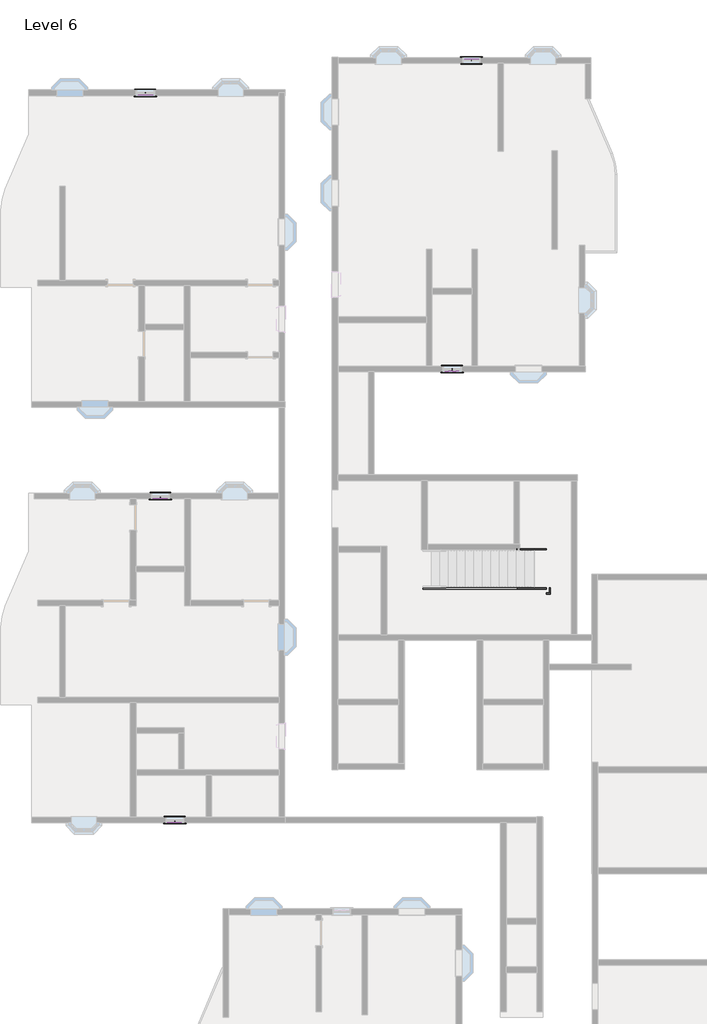
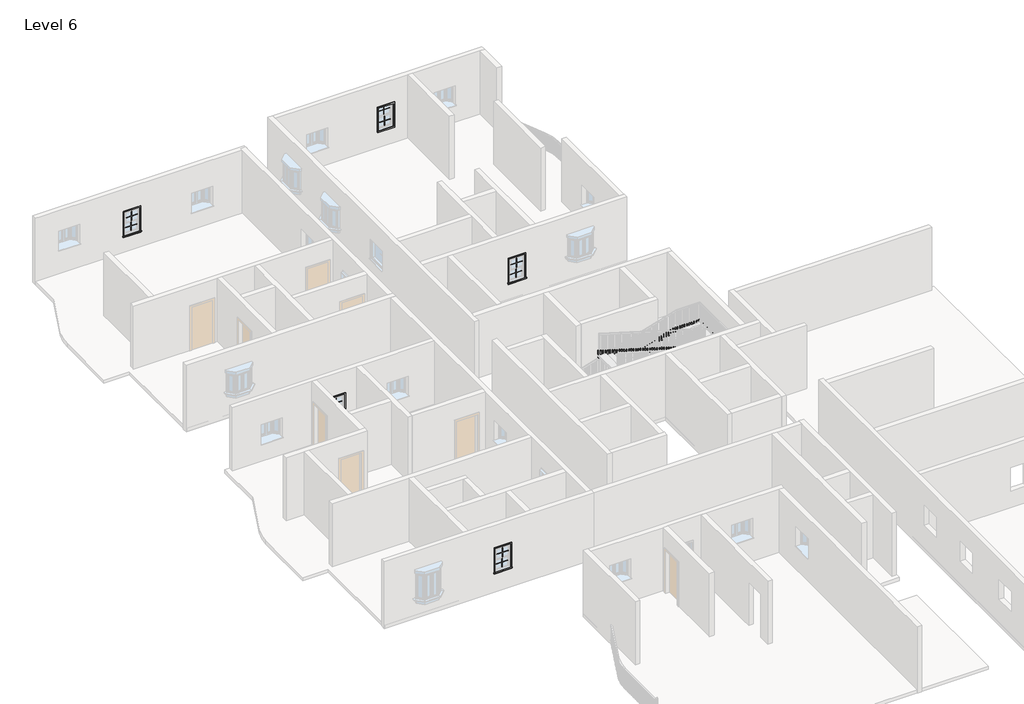
# One storey, part 14 of 14: 20 proxies, 6 members.
"""IFC4 building model written with IfcOpenShell, lengths in millimetres."""

from ifc_helpers import new_model, si_unit, frame, origin, place, context, project, spatial, polyline, outline, extrude, transform, mapped, element, save
from components import muntin_pattern_2x2_muntin_pattern_2x2_c35c595f, trim_window_exterior_flat_with_sill_e38017c9, trim_window_interior_flat_picture_frame_d728ed12

model = new_model("IFC4")

# Units and contexts
model_context = context("Model", 3, world=origin())
ifc_project = project(units=[si_unit("LENGTHUNIT", "METRE", prefix="MILLI")], contexts=[model_context])

# Site, building, storey
site = spatial("IfcSite", under=ifc_project)
building = spatial("IfcBuilding", under=site)
storey = spatial("IfcBuildingStorey", under=building, Name="Level 6", Elevation=15240.0)

# Proxies
placement = place(None, origin())
muntin_pattern_2x2_muntin_pattern_2x2_shape = muntin_pattern_2x2_muntin_pattern_2x2_c35c595f(model_context)
element("IfcBuildingElementProxy", 1, Name="Muntin Pattern_2x2 : Muntin Pattern_2x2", ObjectType="Muntin Pattern_2x2 : Muntin Pattern_2x2", at=placement, inside=storey, context=model_context, shape_type="MappedRepresentation", body=[
    mapped(muntin_pattern_2x2_muntin_pattern_2x2_shape, transform((-14639.3891351, 14368.0833494, 16710.025), x_axis=(-1.0, 0.0, 0.0), y_axis=(0.0, -1.0, 0.0), z_axis=(0.0, 0.0, 1.0))),
])
element("IfcBuildingElementProxy", 2, Name="Muntin Pattern_2x2 : Muntin Pattern_2x2", ObjectType="Muntin Pattern_2x2 : Muntin Pattern_2x2", at=placement, inside=storey, context=model_context, shape_type="MappedRepresentation", body=[
    mapped(muntin_pattern_2x2_muntin_pattern_2x2_shape, transform((-14639.3891351, 14412.5333494, 16230.6), x_axis=(-1.0, 0.0, 0.0), y_axis=(0.0, -1.0, 0.0), z_axis=(0.0, 0.0, 1.0))),
])
element("IfcBuildingElementProxy", 3, Name="Muntin Pattern_2x2 : Muntin Pattern_2x2", ObjectType="Muntin Pattern_2x2 : Muntin Pattern_2x2", at=placement, inside=storey, context=model_context, shape_type="MappedRepresentation", body=[
    mapped(muntin_pattern_2x2_muntin_pattern_2x2_shape, transform((-14125.0391351, 2785.6833494, 16710.025), x_axis=(-1.0, 0.0, 0.0), y_axis=(0.0, -1.0, 0.0), z_axis=(0.0, 0.0, 1.0))),
])
element("IfcBuildingElementProxy", 4, Name="Muntin Pattern_2x2 : Muntin Pattern_2x2", ObjectType="Muntin Pattern_2x2 : Muntin Pattern_2x2", at=placement, inside=storey, context=model_context, shape_type="MappedRepresentation", body=[
    mapped(muntin_pattern_2x2_muntin_pattern_2x2_shape, transform((-14125.0391351, 2830.1333494, 16230.6), x_axis=(-1.0, 0.0, 0.0), y_axis=(0.0, -1.0, 0.0), z_axis=(0.0, 0.0, 1.0))),
])
element("IfcBuildingElementProxy", 5, Name="Muntin Pattern_2x2 : Muntin Pattern_2x2", ObjectType="Muntin Pattern_2x2 : Muntin Pattern_2x2", at=placement, inside=storey, context=model_context, shape_type="MappedRepresentation", body=[
    mapped(muntin_pattern_2x2_muntin_pattern_2x2_shape, transform((-4206.3391351, 18910.0465905, 16710.025), x_axis=(-1.0, 0.0, 0.0), y_axis=(0.0, -1.0, 0.0), z_axis=(0.0, 0.0, 1.0))),
])
element("IfcBuildingElementProxy", 6, Name="Muntin Pattern_2x2 : Muntin Pattern_2x2", ObjectType="Muntin Pattern_2x2 : Muntin Pattern_2x2", at=placement, inside=storey, context=model_context, shape_type="MappedRepresentation", body=[
    mapped(muntin_pattern_2x2_muntin_pattern_2x2_shape, transform((-4206.3391351, 18954.4965905, 16230.6), x_axis=(-1.0, 0.0, 0.0), y_axis=(0.0, -1.0, 0.0), z_axis=(0.0, 0.0, 1.0))),
])
element("IfcBuildingElementProxy", 7, Name="Muntin Pattern_2x2 : Muntin Pattern_2x2", ObjectType="Muntin Pattern_2x2 : Muntin Pattern_2x2", at=placement, inside=storey, context=model_context, shape_type="MappedRepresentation", body=[
    mapped(muntin_pattern_2x2_muntin_pattern_2x2_shape, transform((-3514.1891351, 30066.9965905, 16710.025), x_axis=(1.0, 0.0, 0.0), y_axis=(0.0, 1.0, 0.0), z_axis=(0.0, 0.0, 1.0))),
])
element("IfcBuildingElementProxy", 8, Name="Muntin Pattern_2x2 : Muntin Pattern_2x2", ObjectType="Muntin Pattern_2x2 : Muntin Pattern_2x2", at=placement, inside=storey, context=model_context, shape_type="MappedRepresentation", body=[
    mapped(muntin_pattern_2x2_muntin_pattern_2x2_shape, transform((-3514.1891351, 30022.5465905, 16230.6), x_axis=(1.0, 0.0, 0.0), y_axis=(0.0, 1.0, 0.0), z_axis=(0.0, 0.0, 1.0))),
])
element("IfcBuildingElementProxy", 9, Name="Muntin Pattern_2x2 : Muntin Pattern_2x2", ObjectType="Muntin Pattern_2x2 : Muntin Pattern_2x2", at=placement, inside=storey, context=model_context, shape_type="MappedRepresentation", body=[
    mapped(muntin_pattern_2x2_muntin_pattern_2x2_shape, transform((-15175.9641351, 28782.5833494, 16710.025), x_axis=(-1.0, 0.0, 0.0), y_axis=(0.0, -1.0, 0.0), z_axis=(0.0, 0.0, 1.0))),
])
element("IfcBuildingElementProxy", 10, Name="Muntin Pattern_2x2 : Muntin Pattern_2x2", ObjectType="Muntin Pattern_2x2 : Muntin Pattern_2x2", at=placement, inside=storey, context=model_context, shape_type="MappedRepresentation", body=[
    mapped(muntin_pattern_2x2_muntin_pattern_2x2_shape, transform((-15175.9641351, 28827.0333494, 16230.6), x_axis=(-1.0, 0.0, 0.0), y_axis=(0.0, -1.0, 0.0), z_axis=(0.0, 0.0, 1.0))),
])
trim_window_exterior_flat_with_sill_shape = trim_window_exterior_flat_with_sill_e38017c9(model_context)
element("IfcBuildingElementProxy", 11, Name="Trim-Window-Exterior-Flat : with Sill", ObjectType="Trim-Window-Exterior-Flat : with Sill", at=placement, inside=storey, context=model_context, shape_type="MappedRepresentation", body=[
    mapped(trim_window_exterior_flat_with_sill_shape, transform((-14639.3891351, 14333.1583494, 17221.2), x_axis=(1.0, 0.0, 0.0), y_axis=(0.0, 0.0, 1.0), z_axis=(0.0, -1.0, 0.0))),
])
element("IfcBuildingElementProxy", 12, Name="Trim-Window-Exterior-Flat : with Sill", ObjectType="Trim-Window-Exterior-Flat : with Sill", at=placement, inside=storey, context=model_context, shape_type="MappedRepresentation", body=[
    mapped(trim_window_exterior_flat_with_sill_shape, transform((-14125.0391351, 2750.7583494, 17221.2), x_axis=(1.0, 0.0, 0.0), y_axis=(0.0, 0.0, 1.0), z_axis=(0.0, -1.0, 0.0))),
])
element("IfcBuildingElementProxy", 13, Name="Trim-Window-Exterior-Flat : with Sill", ObjectType="Trim-Window-Exterior-Flat : with Sill", at=placement, inside=storey, context=model_context, shape_type="MappedRepresentation", body=[
    mapped(trim_window_exterior_flat_with_sill_shape, transform((-4206.3391351, 18875.1215905, 17221.2), x_axis=(1.0, 0.0, 0.0), y_axis=(0.0, 0.0, 1.0), z_axis=(0.0, -1.0, 0.0))),
])
element("IfcBuildingElementProxy", 14, Name="Trim-Window-Exterior-Flat : with Sill", ObjectType="Trim-Window-Exterior-Flat : with Sill", at=placement, inside=storey, context=model_context, shape_type="MappedRepresentation", body=[
    mapped(trim_window_exterior_flat_with_sill_shape, transform((-3514.1891351, 30101.9215905, 17221.2), x_axis=(-1.0, 0.0, 0.0), y_axis=(0.0, 0.0, 1.0), z_axis=(0.0, 1.0, 0.0))),
])
element("IfcBuildingElementProxy", 15, Name="Trim-Window-Exterior-Flat : with Sill", ObjectType="Trim-Window-Exterior-Flat : with Sill", at=placement, inside=storey, context=model_context, shape_type="MappedRepresentation", body=[
    mapped(trim_window_exterior_flat_with_sill_shape, transform((-15175.9641351, 28747.6583494, 17221.2), x_axis=(1.0, 0.0, 0.0), y_axis=(0.0, 0.0, 1.0), z_axis=(0.0, -1.0, 0.0))),
])
trim_window_interior_flat_picture_frame_shape = trim_window_interior_flat_picture_frame_d728ed12(model_context)
element("IfcBuildingElementProxy", 16, Name="Trim-Window-Interior-Flat : Picture Frame", ObjectType="Trim-Window-Interior-Flat : Picture Frame", at=placement, inside=storey, context=model_context, shape_type="MappedRepresentation", body=[
    mapped(trim_window_interior_flat_picture_frame_shape, transform((-14639.3891351, 14536.3583494, 17221.2), x_axis=(-1.0, 0.0, 0.0), y_axis=(0.0, 0.0, 1.0), z_axis=(0.0, 1.0, 0.0))),
])
element("IfcBuildingElementProxy", 17, Name="Trim-Window-Interior-Flat : Picture Frame", ObjectType="Trim-Window-Interior-Flat : Picture Frame", at=placement, inside=storey, context=model_context, shape_type="MappedRepresentation", body=[
    mapped(trim_window_interior_flat_picture_frame_shape, transform((-14125.0391351, 2953.9583494, 17221.2), x_axis=(-1.0, 0.0, 0.0), y_axis=(0.0, 0.0, 1.0), z_axis=(0.0, 1.0, 0.0))),
])
element("IfcBuildingElementProxy", 18, Name="Trim-Window-Interior-Flat : Picture Frame", ObjectType="Trim-Window-Interior-Flat : Picture Frame", at=placement, inside=storey, context=model_context, shape_type="MappedRepresentation", body=[
    mapped(trim_window_interior_flat_picture_frame_shape, transform((-4206.3391351, 19078.3215905, 17221.2), x_axis=(-1.0, 0.0, 0.0), y_axis=(0.0, 0.0, 1.0), z_axis=(0.0, 1.0, 0.0))),
])
element("IfcBuildingElementProxy", 19, Name="Trim-Window-Interior-Flat : Picture Frame", ObjectType="Trim-Window-Interior-Flat : Picture Frame", at=placement, inside=storey, context=model_context, shape_type="MappedRepresentation", body=[
    mapped(trim_window_interior_flat_picture_frame_shape, transform((-3514.1891351, 29898.7215905, 17221.2), x_axis=(1.0, 0.0, 0.0), y_axis=(0.0, 0.0, 1.0), z_axis=(0.0, -1.0, 0.0))),
])
element("IfcBuildingElementProxy", 20, Name="Trim-Window-Interior-Flat : Picture Frame", ObjectType="Trim-Window-Interior-Flat : Picture Frame", at=placement, inside=storey, context=model_context, shape_type="MappedRepresentation", body=[
    mapped(trim_window_interior_flat_picture_frame_shape, transform((-15175.9641351, 28950.8583494, 17221.2), x_axis=(-1.0, 0.0, 0.0), y_axis=(0.0, 0.0, 1.0), z_axis=(0.0, 1.0, 0.0))),
])

# Members
element("IfcMember", 21, ObjectType="Stringer - 2\" Width", at=placement, inside=storey, context=model_context, shape_type="SweptSolid", body=[
    extrude(outline(polyline([(15431.5995961, -5254.0891351), (15240.0, -5254.0891351), (15240.0, -4832.019314), (16687.8, -6.019314), (16687.8, -1066.7544553), (15431.5995961, -5254.0891351)])), frame((0.0, 12506.0715905, 0.0), z_axis=(0.0, 1.0, 0.0), x_axis=(0.0, 0.0, 1.0)), (0.0, 0.0, 1.0), 50.8),
])
element("IfcMember", 22, ObjectType="Stringer - 2\" Width", at=placement, inside=storey, context=model_context, shape_type="SweptSolid", body=[
    extrude(outline(polyline([(54.5108649, 12556.8715905), (105.3108649, 12556.8715905), (105.3108649, 9478.4949943), (54.5108649, 9478.4949943), (54.5108649, 12556.8715905)])), frame((0.0, 0.0, 16383.0), z_axis=(0.0, 0.0, 1.0), x_axis=(1.0, 0.0, 0.0)), (0.0, 0.0, 1.0), 304.8),
])
element("IfcMember", 23, ObjectType="Stringer - 2\" Width", at=placement, inside=storey, context=model_context, shape_type="SweptSolid", body=[
    extrude(outline(polyline([(16383.0, 105.3108649), (16475.5395961, 105.3108649), (18083.3595961, -5254.0891351), (17765.1390537, -5254.0891351), (16383.0, -646.9589562), (16383.0, 105.3108649)])), frame((0.0, 9427.6949943, 0.0), z_axis=(0.0, 1.0, 0.0), x_axis=(0.0, 0.0, 1.0)), (0.0, 0.0, 1.0), 50.8),
])
element("IfcMember", 24, ObjectType="Stringer - 2\" Width", at=placement, inside=storey, context=model_context, shape_type="SweptSolid", body=[
    extrude(outline(polyline([(15431.5995961, -5254.0891351), (15240.0, -5254.0891351), (15240.0, -4832.019314), (16469.7390537, -732.8891351), (16687.8, -732.8891351), (16687.8, -1066.7544553), (15431.5995961, -5254.0891351)])), frame((0.0, 11103.4082924, 0.0), z_axis=(0.0, 1.0, 0.0), x_axis=(0.0, 0.0, 1.0)), (0.0, 0.0, 1.0), 50.8),
])
element("IfcMember", 25, ObjectType="Stringer - 2\" Width", at=placement, inside=storey, context=model_context, shape_type="SweptSolid", body=[
    extrude(outline(polyline([(-732.8891351, 11154.2082924), (-682.0891351, 11154.2082924), (-682.0891351, 10976.4082924), (-732.8891351, 10976.4082924), (-732.8891351, 11154.2082924)])), frame((0.0, 0.0, 16383.0), z_axis=(0.0, 0.0, 1.0), x_axis=(1.0, 0.0, 0.0)), (0.0, 0.0, 1.0), 304.8),
])
element("IfcMember", 26, ObjectType="Stringer - 2\" Width", at=placement, inside=storey, context=model_context, shape_type="SweptSolid", body=[
    extrude(outline(polyline([(16393.5390537, -682.0891351), (16711.7595961, -682.0891351), (18083.3595961, -5254.0891351), (17765.1390537, -5254.0891351), (16393.5390537, -682.0891351)])), frame((0.0, 10925.6082924, 0.0), z_axis=(0.0, 1.0, 0.0), x_axis=(0.0, 0.0, 1.0)), (0.0, 0.0, 1.0), 50.8),
])

save(model, "model.ifc")

# Revit data of these elements
# Type "Muntin Pattern_2x2 : Muntin Pattern_2x2"
#   Width [instance default] = 4' - 0"
#   Thickness = 0' - 0 1/2"
#   Height [instance default] = 4' - 0"
#   Distance = 0' - 0 3/4"
#   Interior Material [instance default] = none
#   Exterior Material [instance default] = none
#   Default Elevation = 0
# Type "Trim-Window-Exterior-Flat : with Sill"
#   Trim Width = 0' - 2 1/4"
#   Trim Thickness_Picture Frame = 0' - 1 1/4"
#   Trim Thickness_with Sill = 0' - 0 3/4"
#   Sill Thickness = 0' - 1 1/4"
#   Opening Width [instance default] = 2' - 0"
#   Opening Height [instance default] = 3' - 0"
#   Default Elevation = 4' - 0"
#   Sill = yes
#   Picture Frame = no
#   Trim Material [instance default] = none
# Type "Trim-Window-Interior-Flat : Picture Frame"
#   Trim Thickness_Picture Frame = 0' - 1 1/4"
#   Trim Width = 0' - 2 1/4"
#   Trim Thickness_with Sill = 0' - 0 3/4"
#   Sill Thickness = 0' - 1 1/4"
#   Opening Width [instance default] = 2' - 0"
#   Opening Height [instance default] = 3' - 0"
#   Default Elevation = 4' - 0"
#   Sill = no
#   Picture Frame = yes
#   Trim Material [instance default] = none
# Elements 1, 2, 3, 4, 5, 6, 7, 8, 9, 10 (IfcBuildingElementProxy, "Muntin Pattern_2x2 : Muntin Pattern_2x2")
#   Width = 1' - 8"
#   Height = 1' - 5 1/8"
#   Interior Material = Wood - Stained
#   Exterior Material = Clad - White
#   Phase Created = New Construction
#   Materials on its faces: "Clad - White", "Wood - Stained"
# Elements 11, 12, 13, 14, 15 (IfcBuildingElementProxy, "Trim-Window-Exterior-Flat : with Sill")
#   Opening Width = 2' - 2"
#   Opening Height = 3' - 6"
#   Trim Material = Clad - White
#   Phase Created = New Construction
#   Materials on its faces: "Clad - White"
# Elements 16, 17, 18, 19, 20 (IfcBuildingElementProxy, "Trim-Window-Interior-Flat : Picture Frame")
#   Opening Width = 2' - 2"
#   Opening Height = 3' - 6"
#   Trim Material = Wood - Stained
#   Phase Created = New Construction
#   Materials on its faces: "Wood - Stained"
# Elements 21, 22, 23, 24, 25, 26 (IfcMember, "Stringer - 2\" Width")
#   Phase Created = New Construction
# Materials
#   "Clad - White": class "Wood", colour RGB 242 242 238, transparency 0, Cost = 0
#   "Wood - Stained": class "Wood", colour RGB 224 178 126, transparency 0, Cost = 0
